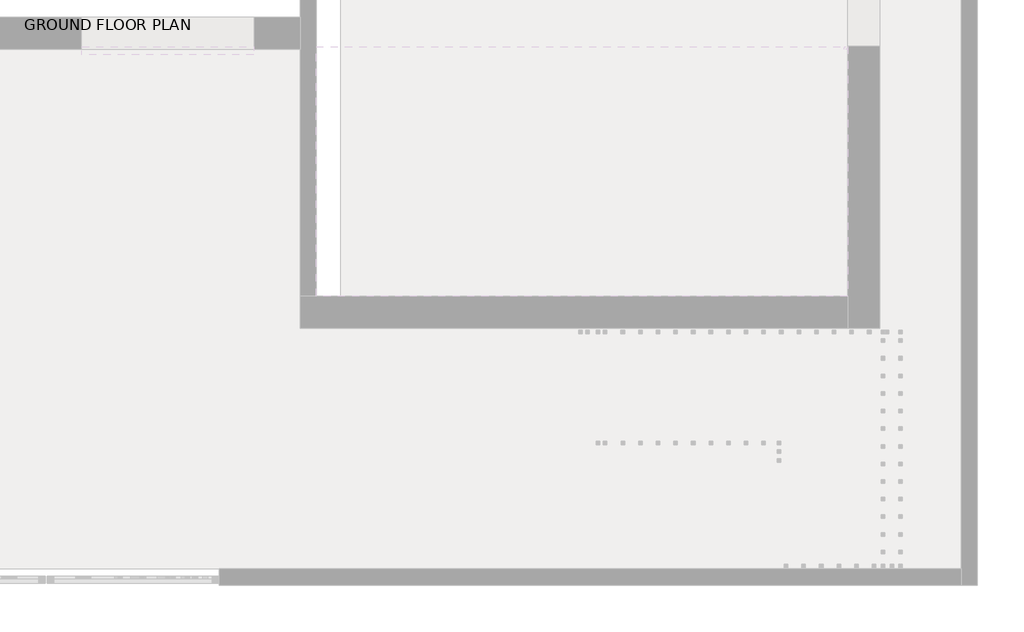
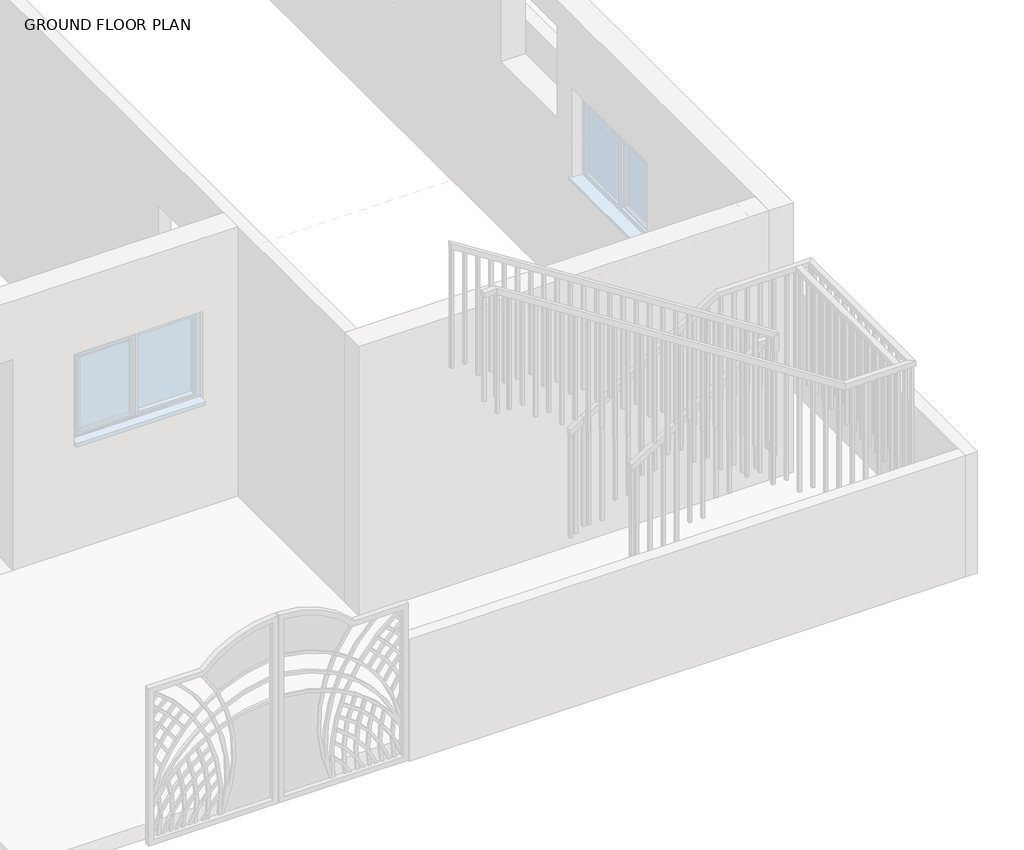
# One storey, part 17 of 23: 2 railings.
"""IFC4 building model written with IfcOpenShell, lengths in millimetres."""

from ifc_helpers import new_model, si_unit, frame, origin, place, context, project, spatial, polyline, outline, extrude, faceted_brep, element, save

model = new_model("IFC4")

# Units and contexts
model_context = context("Model", 3, world=origin())
ifc_project = project(units=[si_unit("LENGTHUNIT", "METRE", prefix="MILLI")], contexts=[model_context])

# Site, building, storey
site = spatial("IfcSite", under=ifc_project)
building = spatial("IfcBuilding", under=site)
storey = spatial("IfcBuildingStorey", under=building, Name="GROUND FLOOR PLAN", Elevation=487.68)

# Railings
placement = place(None, origin())
element("IfcRailing", 1, ObjectType="1100mm", at=placement, inside=storey, context=model_context, shape_type="SolidModel", body=[
    faceted_brep([(-8805.870786, -10220.0521308, 1832.3649576), (-8805.870786, -10220.0521308, 1773.007357), (-8805.870786, -10270.0521308, 1773.007357), (-8805.870786, -10270.0521308, 1832.3649576), (-7409.7306254, -10220.0521308, 2725.6), (-7395.1045513, -10220.0521308, 2675.6), (-7395.1045513, -10270.0521308, 2675.6), (-7409.7306254, -10270.0521308, 2725.6), (-6621.5344696, -10220.0521308, 2725.6), (-6621.5344696, -10220.0521308, 2675.6), (-6671.5344696, -10270.0521308, 2675.6), (-6671.5344696, -10270.0521308, 2725.6), (-6621.5344696, -11933.6860066, 2725.6), (-6621.5344696, -11933.6860066, 2675.6), (-6671.5344696, -11883.6860066, 2675.6), (-6671.5344696, -11883.6860066, 2725.6), (-7155.718398, -11933.6860066, 2725.6), (-7170.3479429, -11933.6860066, 2675.6), (-7170.3479429, -11883.6860066, 2675.6), (-7155.718398, -11883.6860066, 2725.6), (-10457.8773536, -11933.6860066, 4838.88), (-10472.5068984, -11933.6860066, 4788.88), (-10472.5068984, -11883.6860066, 4788.88), (-10457.8773536, -11883.6860066, 4838.88), (-10583.5985666, -11933.6860066, 4838.88), (-10583.5985666, -11883.6860066, 4838.88), (-10583.5985666, -11883.6860066, 4788.88), (-10583.5985666, -11933.6860066, 4788.88)], [[[0, 1, 2, 3]], [[1, 0, 4, 5]], [[2, 1, 5, 6]], [[3, 2, 6, 7]], [[0, 3, 7, 4]], [[5, 4, 8, 9]], [[6, 5, 9, 10]], [[7, 6, 10, 11]], [[4, 7, 11, 8]], [[9, 8, 12, 13]], [[10, 9, 13, 14]], [[11, 10, 14, 15]], [[8, 11, 15, 12]], [[13, 12, 16, 17]], [[14, 13, 17, 18]], [[15, 14, 18, 19]], [[12, 15, 19, 16]], [[17, 16, 20, 21]], [[18, 17, 21, 22]], [[19, 18, 22, 23]], [[16, 19, 23, 20]], [[24, 25, 26, 27]], [[21, 20, 24, 27]], [[22, 21, 27, 26]], [[23, 22, 26, 25]], [[20, 23, 25, 24]]]),
    extrude(outline(polyline([(-10446.5344696, -11921.1860066), (-10471.5344696, -11921.1860066), (-10471.5344696, -11896.1860066), (-10446.5344696, -11896.1860066), (-10446.5344696, -11921.1860066)])), frame((0.0, 0.0, 3738.88), z_axis=(0.0, 0.0, 1.0), x_axis=(1.0, 0.0, 0.0)), (0.0, 0.0, 1.0), 1050.0),
    extrude(outline(polyline([(4692.2622966, -10321.5344696), (4708.2615264, -10346.5344696), (3576.32, -10346.5344696), (3576.32, -10321.5344696), (4692.2622966, -10321.5344696)])), frame((0.0, -11921.1860066, 0.0), z_axis=(0.0, 1.0, 0.0), x_axis=(0.0, 0.0, 1.0)), (0.0, 0.0, 1.0), 25.0),
    extrude(outline(polyline([(4612.2661476, -10196.5344696), (4628.2653774, -10221.5344696), (3576.32, -10221.5344696), (3576.32, -10196.5344696), (4612.2661476, -10196.5344696)])), frame((0.0, -11921.1860066, 0.0), z_axis=(0.0, 1.0, 0.0), x_axis=(0.0, 0.0, 1.0)), (0.0, 0.0, 1.0), 25.0),
    extrude(outline(polyline([(4532.2699985, -10071.5344696), (4548.2692283, -10096.5344696), (3413.76, -10096.5344696), (3413.76, -10071.5344696), (4532.2699985, -10071.5344696)])), frame((0.0, -11921.1860066, 0.0), z_axis=(0.0, 1.0, 0.0), x_axis=(0.0, 0.0, 1.0)), (0.0, 0.0, 1.0), 25.0),
    extrude(outline(polyline([(4452.2738495, -9946.5344696), (4468.2730793, -9971.5344696), (3413.76, -9971.5344696), (3413.76, -9946.5344696), (4452.2738495, -9946.5344696)])), frame((0.0, -11921.1860066, 0.0), z_axis=(0.0, 1.0, 0.0), x_axis=(0.0, 0.0, 1.0)), (0.0, 0.0, 1.0), 25.0),
    extrude(outline(polyline([(4372.2777004, -9821.5344696), (4388.2769302, -9846.5344696), (3251.2, -9846.5344696), (3251.2, -9821.5344696), (4372.2777004, -9821.5344696)])), frame((0.0, -11921.1860066, 0.0), z_axis=(0.0, 1.0, 0.0), x_axis=(0.0, 0.0, 1.0)), (0.0, 0.0, 1.0), 25.0),
    extrude(outline(polyline([(4292.2815514, -9696.5344696), (4308.2807812, -9721.5344696), (3251.2, -9721.5344696), (3251.2, -9696.5344696), (4292.2815514, -9696.5344696)])), frame((0.0, -11921.1860066, 0.0), z_axis=(0.0, 1.0, 0.0), x_axis=(0.0, 0.0, 1.0)), (0.0, 0.0, 1.0), 25.0),
    extrude(outline(polyline([(4212.2854023, -9571.5344696), (4228.2846321, -9596.5344696), (3088.64, -9596.5344696), (3088.64, -9571.5344696), (4212.2854023, -9571.5344696)])), frame((0.0, -11921.1860066, 0.0), z_axis=(0.0, 1.0, 0.0), x_axis=(0.0, 0.0, 1.0)), (0.0, 0.0, 1.0), 25.0),
    extrude(outline(polyline([(4132.2892533, -9446.5344696), (4148.2884831, -9471.5344696), (3088.64, -9471.5344696), (3088.64, -9446.5344696), (4132.2892533, -9446.5344696)])), frame((0.0, -11921.1860066, 0.0), z_axis=(0.0, 1.0, 0.0), x_axis=(0.0, 0.0, 1.0)), (0.0, 0.0, 1.0), 25.0),
    extrude(outline(polyline([(4052.2931042, -9321.5344696), (4068.292334, -9346.5344696), (2926.08, -9346.5344696), (2926.08, -9321.5344696), (4052.2931042, -9321.5344696)])), frame((0.0, -11921.1860066, 0.0), z_axis=(0.0, 1.0, 0.0), x_axis=(0.0, 0.0, 1.0)), (0.0, 0.0, 1.0), 25.0),
    extrude(outline(polyline([(3972.2969552, -9196.5344696), (3988.296185, -9221.5344696), (2926.08, -9221.5344696), (2926.08, -9196.5344696), (3972.2969552, -9196.5344696)])), frame((0.0, -11921.1860066, 0.0), z_axis=(0.0, 1.0, 0.0), x_axis=(0.0, 0.0, 1.0)), (0.0, 0.0, 1.0), 25.0),
    extrude(outline(polyline([(3892.3008061, -9071.5344696), (3908.3000359, -9096.5344696), (2763.52, -9096.5344696), (2763.52, -9071.5344696), (3892.3008061, -9071.5344696)])), frame((0.0, -11921.1860066, 0.0), z_axis=(0.0, 1.0, 0.0), x_axis=(0.0, 0.0, 1.0)), (0.0, 0.0, 1.0), 25.0),
    extrude(outline(polyline([(3812.3046571, -8946.5344696), (3828.3038869, -8971.5344696), (2763.52, -8971.5344696), (2763.52, -8946.5344696), (3812.3046571, -8946.5344696)])), frame((0.0, -11921.1860066, 0.0), z_axis=(0.0, 1.0, 0.0), x_axis=(0.0, 0.0, 1.0)), (0.0, 0.0, 1.0), 25.0),
    extrude(outline(polyline([(3732.308508, -8821.5344696), (3748.3077378, -8846.5344696), (2600.96, -8846.5344696), (2600.96, -8821.5344696), (3732.308508, -8821.5344696)])), frame((0.0, -11921.1860066, 0.0), z_axis=(0.0, 1.0, 0.0), x_axis=(0.0, 0.0, 1.0)), (0.0, 0.0, 1.0), 25.0),
    extrude(outline(polyline([(3652.312359, -8696.5344696), (3668.3115888, -8721.5344696), (2600.96, -8721.5344696), (2600.96, -8696.5344696), (3652.312359, -8696.5344696)])), frame((0.0, -11921.1860066, 0.0), z_axis=(0.0, 1.0, 0.0), x_axis=(0.0, 0.0, 1.0)), (0.0, 0.0, 1.0), 25.0),
    extrude(outline(polyline([(3572.3162099, -8571.5344696), (3588.3154397, -8596.5344696), (2438.4, -8596.5344696), (2438.4, -8571.5344696), (3572.3162099, -8571.5344696)])), frame((0.0, -11921.1860066, 0.0), z_axis=(0.0, 1.0, 0.0), x_axis=(0.0, 0.0, 1.0)), (0.0, 0.0, 1.0), 25.0),
    extrude(outline(polyline([(3492.3200609, -8446.5344696), (3508.3192907, -8471.5344696), (2438.4, -8471.5344696), (2438.4, -8446.5344696), (3492.3200609, -8446.5344696)])), frame((0.0, -11921.1860066, 0.0), z_axis=(0.0, 1.0, 0.0), x_axis=(0.0, 0.0, 1.0)), (0.0, 0.0, 1.0), 25.0),
    extrude(outline(polyline([(3412.3239118, -8321.5344696), (3428.3231416, -8346.5344696), (2275.84, -8346.5344696), (2275.84, -8321.5344696), (3412.3239118, -8321.5344696)])), frame((0.0, -11921.1860066, 0.0), z_axis=(0.0, 1.0, 0.0), x_axis=(0.0, 0.0, 1.0)), (0.0, 0.0, 1.0), 25.0),
    extrude(outline(polyline([(3332.3277628, -8196.5344696), (3348.3269926, -8221.5344696), (2275.84, -8221.5344696), (2275.84, -8196.5344696), (3332.3277628, -8196.5344696)])), frame((0.0, -11921.1860066, 0.0), z_axis=(0.0, 1.0, 0.0), x_axis=(0.0, 0.0, 1.0)), (0.0, 0.0, 1.0), 25.0),
    extrude(outline(polyline([(3252.3316137, -8071.5344696), (3268.3308435, -8096.5344696), (2113.28, -8096.5344696), (2113.28, -8071.5344696), (3252.3316137, -8071.5344696)])), frame((0.0, -11921.1860066, 0.0), z_axis=(0.0, 1.0, 0.0), x_axis=(0.0, 0.0, 1.0)), (0.0, 0.0, 1.0), 25.0),
    extrude(outline(polyline([(3172.3354647, -7946.5344696), (3188.3346945, -7971.5344696), (2113.28, -7971.5344696), (2113.28, -7946.5344696), (3172.3354647, -7946.5344696)])), frame((0.0, -11921.1860066, 0.0), z_axis=(0.0, 1.0, 0.0), x_axis=(0.0, 0.0, 1.0)), (0.0, 0.0, 1.0), 25.0),
    extrude(outline(polyline([(3092.4129874, -7821.5344696), (3108.4077111, -7846.5344696), (1950.72, -7846.5344696), (1950.72, -7821.5344696), (3092.4129874, -7821.5344696)])), frame((0.0, -11921.1860066, 0.0), z_axis=(0.0, 1.0, 0.0), x_axis=(0.0, 0.0, 1.0)), (0.0, 0.0, 1.0), 25.0),
    extrude(outline(polyline([(3012.4393691, -7696.5344696), (3028.4340928, -7721.5344696), (1950.72, -7721.5344696), (1950.72, -7696.5344696), (3012.4393691, -7696.5344696)])), frame((0.0, -11921.1860066, 0.0), z_axis=(0.0, 1.0, 0.0), x_axis=(0.0, 0.0, 1.0)), (0.0, 0.0, 1.0), 25.0),
    extrude(outline(polyline([(2932.4657508, -7571.5344696), (2948.4604745, -7596.5344696), (1788.16, -7596.5344696), (1788.16, -7571.5344696), (2932.4657508, -7571.5344696)])), frame((0.0, -11921.1860066, 0.0), z_axis=(0.0, 1.0, 0.0), x_axis=(0.0, 0.0, 1.0)), (0.0, 0.0, 1.0), 25.0),
    extrude(outline(polyline([(2852.4921325, -7446.5344696), (2868.4868562, -7471.5344696), (1788.16, -7471.5344696), (1788.16, -7446.5344696), (2852.4921325, -7446.5344696)])), frame((0.0, -11921.1860066, 0.0), z_axis=(0.0, 1.0, 0.0), x_axis=(0.0, 0.0, 1.0)), (0.0, 0.0, 1.0), 25.0),
    extrude(outline(polyline([(2772.3547194, -7321.5344696), (2788.3539492, -7346.5344696), (1625.6, -7346.5344696), (1625.6, -7321.5344696), (2772.3547194, -7321.5344696)])), frame((0.0, -11921.1860066, 0.0), z_axis=(0.0, 1.0, 0.0), x_axis=(0.0, 0.0, 1.0)), (0.0, 0.0, 1.0), 25.0),
    extrude(outline(polyline([(2692.3585703, -7196.5344696), (2708.3578001, -7221.5344696), (1625.6, -7221.5344696), (1625.6, -7196.5344696), (2692.3585703, -7196.5344696)])), frame((0.0, -11921.1860066, 0.0), z_axis=(0.0, 1.0, 0.0), x_axis=(0.0, 0.0, 1.0)), (0.0, 0.0, 1.0), 25.0),
    extrude(outline(polyline([(-7071.5344696, -11921.1860066), (-7096.5344696, -11921.1860066), (-7096.5344696, -11896.1860066), (-7071.5344696, -11896.1860066), (-7071.5344696, -11921.1860066)])), frame((0.0, 0.0, 1625.6), z_axis=(0.0, 0.0, 1.0), x_axis=(1.0, 0.0, 0.0)), (0.0, 0.0, 1.0), 1050.0),
    extrude(outline(polyline([(-6946.5344696, -11921.1860066), (-6971.5344696, -11921.1860066), (-6971.5344696, -11896.1860066), (-6946.5344696, -11896.1860066), (-6946.5344696, -11921.1860066)])), frame((0.0, 0.0, 1625.6), z_axis=(0.0, 0.0, 1.0), x_axis=(1.0, 0.0, 0.0)), (0.0, 0.0, 1.0), 1050.0),
    extrude(outline(polyline([(-6821.5344696, -11921.1860066), (-6846.5344696, -11921.1860066), (-6846.5344696, -11896.1860066), (-6821.5344696, -11896.1860066), (-6821.5344696, -11921.1860066)])), frame((0.0, 0.0, 1625.6), z_axis=(0.0, 0.0, 1.0), x_axis=(1.0, 0.0, 0.0)), (0.0, 0.0, 1.0), 1050.0),
    extrude(outline(polyline([(-6696.5344696, -11921.1860066), (-6721.5344696, -11921.1860066), (-6721.5344696, -11896.1860066), (-6696.5344696, -11896.1860066), (-6696.5344696, -11921.1860066)])), frame((0.0, 0.0, 1625.6), z_axis=(0.0, 0.0, 1.0), x_axis=(1.0, 0.0, 0.0)), (0.0, 0.0, 1.0), 1050.0),
    extrude(outline(polyline([(-6634.0344696, -11795.0521308), (-6634.0344696, -11820.0521308), (-6659.0344696, -11820.0521308), (-6659.0344696, -11795.0521308), (-6634.0344696, -11795.0521308)])), frame((0.0, 0.0, 1625.6), z_axis=(0.0, 0.0, 1.0), x_axis=(1.0, 0.0, 0.0)), (0.0, 0.0, 1.0), 1050.0),
    extrude(outline(polyline([(-6634.0344696, -11670.0521308), (-6634.0344696, -11695.0521308), (-6659.0344696, -11695.0521308), (-6659.0344696, -11670.0521308), (-6634.0344696, -11670.0521308)])), frame((0.0, 0.0, 1625.6), z_axis=(0.0, 0.0, 1.0), x_axis=(1.0, 0.0, 0.0)), (0.0, 0.0, 1.0), 1050.0),
    extrude(outline(polyline([(-6634.0344696, -11545.0521308), (-6634.0344696, -11570.0521308), (-6659.0344696, -11570.0521308), (-6659.0344696, -11545.0521308), (-6634.0344696, -11545.0521308)])), frame((0.0, 0.0, 1625.6), z_axis=(0.0, 0.0, 1.0), x_axis=(1.0, 0.0, 0.0)), (0.0, 0.0, 1.0), 1050.0),
    extrude(outline(polyline([(-6634.0344696, -11420.0521308), (-6634.0344696, -11445.0521308), (-6659.0344696, -11445.0521308), (-6659.0344696, -11420.0521308), (-6634.0344696, -11420.0521308)])), frame((0.0, 0.0, 1625.6), z_axis=(0.0, 0.0, 1.0), x_axis=(1.0, 0.0, 0.0)), (0.0, 0.0, 1.0), 1050.0),
    extrude(outline(polyline([(-6634.0344696, -11295.0521308), (-6634.0344696, -11320.0521308), (-6659.0344696, -11320.0521308), (-6659.0344696, -11295.0521308), (-6634.0344696, -11295.0521308)])), frame((0.0, 0.0, 1625.6), z_axis=(0.0, 0.0, 1.0), x_axis=(1.0, 0.0, 0.0)), (0.0, 0.0, 1.0), 1050.0),
    extrude(outline(polyline([(-6634.0344696, -11170.0521308), (-6634.0344696, -11195.0521308), (-6659.0344696, -11195.0521308), (-6659.0344696, -11170.0521308), (-6634.0344696, -11170.0521308)])), frame((0.0, 0.0, 1625.6), z_axis=(0.0, 0.0, 1.0), x_axis=(1.0, 0.0, 0.0)), (0.0, 0.0, 1.0), 1050.0),
    extrude(outline(polyline([(-6634.0344696, -11045.0521308), (-6634.0344696, -11070.0521308), (-6659.0344696, -11070.0521308), (-6659.0344696, -11045.0521308), (-6634.0344696, -11045.0521308)])), frame((0.0, 0.0, 1625.6), z_axis=(0.0, 0.0, 1.0), x_axis=(1.0, 0.0, 0.0)), (0.0, 0.0, 1.0), 1050.0),
    extrude(outline(polyline([(-6634.0344696, -10920.0521308), (-6634.0344696, -10945.0521308), (-6659.0344696, -10945.0521308), (-6659.0344696, -10920.0521308), (-6634.0344696, -10920.0521308)])), frame((0.0, 0.0, 1625.6), z_axis=(0.0, 0.0, 1.0), x_axis=(1.0, 0.0, 0.0)), (0.0, 0.0, 1.0), 1050.0),
    extrude(outline(polyline([(-6634.0344696, -10795.0521308), (-6634.0344696, -10820.0521308), (-6659.0344696, -10820.0521308), (-6659.0344696, -10795.0521308), (-6634.0344696, -10795.0521308)])), frame((0.0, 0.0, 1625.6), z_axis=(0.0, 0.0, 1.0), x_axis=(1.0, 0.0, 0.0)), (0.0, 0.0, 1.0), 1050.0),
    extrude(outline(polyline([(-6634.0344696, -10670.0521308), (-6634.0344696, -10695.0521308), (-6659.0344696, -10695.0521308), (-6659.0344696, -10670.0521308), (-6634.0344696, -10670.0521308)])), frame((0.0, 0.0, 1625.6), z_axis=(0.0, 0.0, 1.0), x_axis=(1.0, 0.0, 0.0)), (0.0, 0.0, 1.0), 1050.0),
    extrude(outline(polyline([(-6634.0344696, -10545.0521308), (-6634.0344696, -10570.0521308), (-6659.0344696, -10570.0521308), (-6659.0344696, -10545.0521308), (-6634.0344696, -10545.0521308)])), frame((0.0, 0.0, 1625.6), z_axis=(0.0, 0.0, 1.0), x_axis=(1.0, 0.0, 0.0)), (0.0, 0.0, 1.0), 1050.0),
    extrude(outline(polyline([(-6634.0344696, -10420.0521308), (-6634.0344696, -10445.0521308), (-6659.0344696, -10445.0521308), (-6659.0344696, -10420.0521308), (-6634.0344696, -10420.0521308)])), frame((0.0, 0.0, 1625.6), z_axis=(0.0, 0.0, 1.0), x_axis=(1.0, 0.0, 0.0)), (0.0, 0.0, 1.0), 1050.0),
    extrude(outline(polyline([(-6634.0344696, -10295.0521308), (-6634.0344696, -10320.0521308), (-6659.0344696, -10320.0521308), (-6659.0344696, -10295.0521308), (-6634.0344696, -10295.0521308)])), frame((0.0, 0.0, 1625.6), z_axis=(0.0, 0.0, 1.0), x_axis=(1.0, 0.0, 0.0)), (0.0, 0.0, 1.0), 1050.0),
    extrude(outline(polyline([(-6755.870786, -10232.5521308), (-6730.870786, -10232.5521308), (-6730.870786, -10257.5521308), (-6755.870786, -10257.5521308), (-6755.870786, -10232.5521308)])), frame((0.0, 0.0, 1625.6), z_axis=(0.0, 0.0, 1.0), x_axis=(1.0, 0.0, 0.0)), (0.0, 0.0, 1.0), 1050.0),
    extrude(outline(polyline([(-6880.870786, -10232.5521308), (-6855.870786, -10232.5521308), (-6855.870786, -10257.5521308), (-6880.870786, -10257.5521308), (-6880.870786, -10232.5521308)])), frame((0.0, 0.0, 1625.6), z_axis=(0.0, 0.0, 1.0), x_axis=(1.0, 0.0, 0.0)), (0.0, 0.0, 1.0), 1050.0),
    extrude(outline(polyline([(-7005.870786, -10232.5521308), (-6980.870786, -10232.5521308), (-6980.870786, -10257.5521308), (-7005.870786, -10257.5521308), (-7005.870786, -10232.5521308)])), frame((0.0, 0.0, 1625.6), z_axis=(0.0, 0.0, 1.0), x_axis=(1.0, 0.0, 0.0)), (0.0, 0.0, 1.0), 1050.0),
    extrude(outline(polyline([(-7130.870786, -10232.5521308), (-7105.870786, -10232.5521308), (-7105.870786, -10257.5521308), (-7130.870786, -10257.5521308), (-7130.870786, -10232.5521308)])), frame((0.0, 0.0, 1625.6), z_axis=(0.0, 0.0, 1.0), x_axis=(1.0, 0.0, 0.0)), (0.0, 0.0, 1.0), 1050.0),
    extrude(outline(polyline([(-7255.870786, -10232.5521308), (-7230.870786, -10232.5521308), (-7230.870786, -10257.5521308), (-7255.870786, -10257.5521308), (-7255.870786, -10232.5521308)])), frame((0.0, 0.0, 1625.6), z_axis=(0.0, 0.0, 1.0), x_axis=(1.0, 0.0, 0.0)), (0.0, 0.0, 1.0), 1050.0),
    extrude(outline(polyline([(-7380.870786, -10232.5521308), (-7355.870786, -10232.5521308), (-7355.870786, -10257.5521308), (-7380.870786, -10257.5521308), (-7380.870786, -10232.5521308)])), frame((0.0, 0.0, 1625.6), z_axis=(0.0, 0.0, 1.0), x_axis=(1.0, 0.0, 0.0)), (0.0, 0.0, 1.0), 1050.0),
    extrude(outline(polyline([(1463.04, -7505.870786), (1463.04, -7480.870786), (2620.7277111, -7480.870786), (2604.7329874, -7505.870786), (1463.04, -7505.870786)])), frame((0.0, -10257.5521308, 0.0), z_axis=(0.0, 1.0, 0.0), x_axis=(0.0, 0.0, 1.0)), (0.0, 0.0, 1.0), 25.0),
    extrude(outline(polyline([(1463.04, -7630.870786), (1463.04, -7605.870786), (2540.7540928, -7605.870786), (2524.7593691, -7630.870786), (1463.04, -7630.870786)])), frame((0.0, -10257.5521308, 0.0), z_axis=(0.0, 1.0, 0.0), x_axis=(0.0, 0.0, 1.0)), (0.0, 0.0, 1.0), 25.0),
    extrude(outline(polyline([(1300.48, -7755.870786), (1300.48, -7730.870786), (2460.7804745, -7730.870786), (2444.7857508, -7755.870786), (1300.48, -7755.870786)])), frame((0.0, -10257.5521308, 0.0), z_axis=(0.0, 1.0, 0.0), x_axis=(0.0, 0.0, 1.0)), (0.0, 0.0, 1.0), 25.0),
    extrude(outline(polyline([(1300.48, -7880.870786), (1300.48, -7855.870786), (2380.8068562, -7855.870786), (2364.8121325, -7880.870786), (1300.48, -7880.870786)])), frame((0.0, -10257.5521308, 0.0), z_axis=(0.0, 1.0, 0.0), x_axis=(0.0, 0.0, 1.0)), (0.0, 0.0, 1.0), 25.0),
    extrude(outline(polyline([(1137.92, -8005.870786), (1137.92, -7980.870786), (2300.8332379, -7980.870786), (2284.8385142, -8005.870786), (1137.92, -8005.870786)])), frame((0.0, -10257.5521308, 0.0), z_axis=(0.0, 1.0, 0.0), x_axis=(0.0, 0.0, 1.0)), (0.0, 0.0, 1.0), 25.0),
    extrude(outline(polyline([(1137.92, -8130.870786), (1137.92, -8105.870786), (2220.8596196, -8105.870786), (2204.8648959, -8130.870786), (1137.92, -8130.870786)])), frame((0.0, -10257.5521308, 0.0), z_axis=(0.0, 1.0, 0.0), x_axis=(0.0, 0.0, 1.0)), (0.0, 0.0, 1.0), 25.0),
    extrude(outline(polyline([(975.36, -8255.870786), (975.36, -8230.870786), (2140.8860012, -8230.870786), (2124.8912776, -8255.870786), (975.36, -8255.870786)])), frame((0.0, -10257.5521308, 0.0), z_axis=(0.0, 1.0, 0.0), x_axis=(0.0, 0.0, 1.0)), (0.0, 0.0, 1.0), 25.0),
    extrude(outline(polyline([(975.36, -8380.870786), (975.36, -8355.870786), (2060.9123829, -8355.870786), (2044.9176593, -8380.870786), (975.36, -8380.870786)])), frame((0.0, -10257.5521308, 0.0), z_axis=(0.0, 1.0, 0.0), x_axis=(0.0, 0.0, 1.0)), (0.0, 0.0, 1.0), 25.0),
    extrude(outline(polyline([(812.8, -8505.870786), (812.8, -8480.870786), (1980.9387646, -8480.870786), (1964.944041, -8505.870786), (812.8, -8505.870786)])), frame((0.0, -10257.5521308, 0.0), z_axis=(0.0, 1.0, 0.0), x_axis=(0.0, 0.0, 1.0)), (0.0, 0.0, 1.0), 25.0),
    extrude(outline(polyline([(812.8, -8630.870786), (812.8, -8605.870786), (1900.9651463, -8605.870786), (1884.9704227, -8630.870786), (812.8, -8630.870786)])), frame((0.0, -10257.5521308, 0.0), z_axis=(0.0, 1.0, 0.0), x_axis=(0.0, 0.0, 1.0)), (0.0, 0.0, 1.0), 25.0),
    extrude(outline(polyline([(772.3517667, -8755.870786), (772.3517667, -8730.870786), (1820.991528, -8730.870786), (1804.9968044, -8755.870786), (772.3517667, -8755.870786)])), frame((0.0, -10257.5521308, 0.0), z_axis=(0.0, 1.0, 0.0), x_axis=(0.0, 0.0, 1.0)), (0.0, 0.0, 1.0), 25.0),
    extrude(outline(polyline([(-6634.0344696, -11896.1860066), (-6634.0344696, -11921.1860066), (-6659.0344696, -11921.1860066), (-6659.0344696, -11896.1860066), (-6634.0344696, -11896.1860066)])), frame((0.0, 0.0, 1625.6), z_axis=(0.0, 0.0, 1.0), x_axis=(1.0, 0.0, 0.0)), (0.0, 0.0, 1.0), 1050.0),
    extrude(outline(polyline([(-6659.0344696, -10232.5521308), (-6634.0344696, -10232.5521308), (-6634.0344696, -10257.5521308), (-6659.0344696, -10257.5521308), (-6659.0344696, -10232.5521308)])), frame((0.0, 0.0, 1625.6), z_axis=(0.0, 0.0, 1.0), x_axis=(1.0, 0.0, 0.0)), (0.0, 0.0, 1.0), 1050.0),
    extrude(outline(polyline([(-10558.5985666, -11921.1860066), (-10583.5985666, -11921.1860066), (-10583.5985666, -11896.1860066), (-10558.5985666, -11896.1860066), (-10558.5985666, -11921.1860066)])), frame((0.0, 0.0, 3738.88), z_axis=(0.0, 0.0, 1.0), x_axis=(1.0, 0.0, 0.0)), (0.0, 0.0, 1.0), 1050.0),
    extrude(outline(polyline([(740.3623194, -8805.870786), (740.3623194, -8780.870786), (1789.0020807, -8780.870786), (1773.007357, -8805.870786), (740.3623194, -8805.870786)])), frame((0.0, -10257.5521308, 0.0), z_axis=(0.0, 1.0, 0.0), x_axis=(0.0, 0.0, 1.0)), (0.0, 0.0, 1.0), 25.0),
])
element("IfcRailing", 2, ObjectType="1100mm", at=placement, inside=storey, context=model_context, shape_type="SolidModel", body=[
    faceted_brep([(-8805.870786, -10220.0521308, 1832.3649576), (-8805.870786, -10220.0521308, 1773.007357), (-8805.870786, -10270.0521308, 1773.007357), (-8805.870786, -10270.0521308, 1832.3649576), (-7409.7306254, -10220.0521308, 2725.6), (-7395.1045513, -10220.0521308, 2675.6), (-7395.1045513, -10270.0521308, 2675.6), (-7409.7306254, -10270.0521308, 2725.6), (-6621.5344696, -10220.0521308, 2725.6), (-6621.5344696, -10220.0521308, 2675.6), (-6671.5344696, -10270.0521308, 2675.6), (-6671.5344696, -10270.0521308, 2725.6), (-6621.5344696, -11933.6860066, 2725.6), (-6621.5344696, -11933.6860066, 2675.6), (-6671.5344696, -11883.6860066, 2675.6), (-6671.5344696, -11883.6860066, 2725.6), (-7155.718398, -11933.6860066, 2725.6), (-7170.3479429, -11933.6860066, 2675.6), (-7170.3479429, -11883.6860066, 2675.6), (-7155.718398, -11883.6860066, 2725.6), (-10457.8773536, -11933.6860066, 4838.88), (-10472.5068984, -11933.6860066, 4788.88), (-10472.5068984, -11883.6860066, 4788.88), (-10457.8773536, -11883.6860066, 4838.88), (-10583.5985666, -11933.6860066, 4838.88), (-10583.5985666, -11883.6860066, 4838.88), (-10583.5985666, -11883.6860066, 4788.88), (-10583.5985666, -11933.6860066, 4788.88)], [[[0, 1, 2, 3]], [[1, 0, 4, 5]], [[2, 1, 5, 6]], [[3, 2, 6, 7]], [[0, 3, 7, 4]], [[5, 4, 8, 9]], [[6, 5, 9, 10]], [[7, 6, 10, 11]], [[4, 7, 11, 8]], [[9, 8, 12, 13]], [[10, 9, 13, 14]], [[11, 10, 14, 15]], [[8, 11, 15, 12]], [[13, 12, 16, 17]], [[14, 13, 17, 18]], [[15, 14, 18, 19]], [[12, 15, 19, 16]], [[17, 16, 20, 21]], [[18, 17, 21, 22]], [[19, 18, 22, 23]], [[16, 19, 23, 20]], [[24, 25, 26, 27]], [[21, 20, 24, 27]], [[22, 21, 27, 26]], [[23, 22, 26, 25]], [[20, 23, 25, 24]]]),
    extrude(outline(polyline([(-10446.5344696, -11921.1860066), (-10471.5344696, -11921.1860066), (-10471.5344696, -11896.1860066), (-10446.5344696, -11896.1860066), (-10446.5344696, -11921.1860066)])), frame((0.0, 0.0, 3738.88), z_axis=(0.0, 0.0, 1.0), x_axis=(1.0, 0.0, 0.0)), (0.0, 0.0, 1.0), 1050.0),
    extrude(outline(polyline([(4692.2622966, -10321.5344696), (4708.2615264, -10346.5344696), (3576.32, -10346.5344696), (3576.32, -10321.5344696), (4692.2622966, -10321.5344696)])), frame((0.0, -11921.1860066, 0.0), z_axis=(0.0, 1.0, 0.0), x_axis=(0.0, 0.0, 1.0)), (0.0, 0.0, 1.0), 25.0),
    extrude(outline(polyline([(4612.2661476, -10196.5344696), (4628.2653774, -10221.5344696), (3576.32, -10221.5344696), (3576.32, -10196.5344696), (4612.2661476, -10196.5344696)])), frame((0.0, -11921.1860066, 0.0), z_axis=(0.0, 1.0, 0.0), x_axis=(0.0, 0.0, 1.0)), (0.0, 0.0, 1.0), 25.0),
    extrude(outline(polyline([(4532.2699985, -10071.5344696), (4548.2692283, -10096.5344696), (3413.76, -10096.5344696), (3413.76, -10071.5344696), (4532.2699985, -10071.5344696)])), frame((0.0, -11921.1860066, 0.0), z_axis=(0.0, 1.0, 0.0), x_axis=(0.0, 0.0, 1.0)), (0.0, 0.0, 1.0), 25.0),
    extrude(outline(polyline([(4452.2738495, -9946.5344696), (4468.2730793, -9971.5344696), (3413.76, -9971.5344696), (3413.76, -9946.5344696), (4452.2738495, -9946.5344696)])), frame((0.0, -11921.1860066, 0.0), z_axis=(0.0, 1.0, 0.0), x_axis=(0.0, 0.0, 1.0)), (0.0, 0.0, 1.0), 25.0),
    extrude(outline(polyline([(4372.2777004, -9821.5344696), (4388.2769302, -9846.5344696), (3251.2, -9846.5344696), (3251.2, -9821.5344696), (4372.2777004, -9821.5344696)])), frame((0.0, -11921.1860066, 0.0), z_axis=(0.0, 1.0, 0.0), x_axis=(0.0, 0.0, 1.0)), (0.0, 0.0, 1.0), 25.0),
    extrude(outline(polyline([(4292.2815514, -9696.5344696), (4308.2807812, -9721.5344696), (3251.2, -9721.5344696), (3251.2, -9696.5344696), (4292.2815514, -9696.5344696)])), frame((0.0, -11921.1860066, 0.0), z_axis=(0.0, 1.0, 0.0), x_axis=(0.0, 0.0, 1.0)), (0.0, 0.0, 1.0), 25.0),
    extrude(outline(polyline([(4212.2854023, -9571.5344696), (4228.2846321, -9596.5344696), (3088.64, -9596.5344696), (3088.64, -9571.5344696), (4212.2854023, -9571.5344696)])), frame((0.0, -11921.1860066, 0.0), z_axis=(0.0, 1.0, 0.0), x_axis=(0.0, 0.0, 1.0)), (0.0, 0.0, 1.0), 25.0),
    extrude(outline(polyline([(4132.2892533, -9446.5344696), (4148.2884831, -9471.5344696), (3088.64, -9471.5344696), (3088.64, -9446.5344696), (4132.2892533, -9446.5344696)])), frame((0.0, -11921.1860066, 0.0), z_axis=(0.0, 1.0, 0.0), x_axis=(0.0, 0.0, 1.0)), (0.0, 0.0, 1.0), 25.0),
    extrude(outline(polyline([(4052.2931042, -9321.5344696), (4068.292334, -9346.5344696), (2926.08, -9346.5344696), (2926.08, -9321.5344696), (4052.2931042, -9321.5344696)])), frame((0.0, -11921.1860066, 0.0), z_axis=(0.0, 1.0, 0.0), x_axis=(0.0, 0.0, 1.0)), (0.0, 0.0, 1.0), 25.0),
    extrude(outline(polyline([(3972.2969552, -9196.5344696), (3988.296185, -9221.5344696), (2926.08, -9221.5344696), (2926.08, -9196.5344696), (3972.2969552, -9196.5344696)])), frame((0.0, -11921.1860066, 0.0), z_axis=(0.0, 1.0, 0.0), x_axis=(0.0, 0.0, 1.0)), (0.0, 0.0, 1.0), 25.0),
    extrude(outline(polyline([(3892.3008061, -9071.5344696), (3908.3000359, -9096.5344696), (2763.52, -9096.5344696), (2763.52, -9071.5344696), (3892.3008061, -9071.5344696)])), frame((0.0, -11921.1860066, 0.0), z_axis=(0.0, 1.0, 0.0), x_axis=(0.0, 0.0, 1.0)), (0.0, 0.0, 1.0), 25.0),
    extrude(outline(polyline([(3812.3046571, -8946.5344696), (3828.3038869, -8971.5344696), (2763.52, -8971.5344696), (2763.52, -8946.5344696), (3812.3046571, -8946.5344696)])), frame((0.0, -11921.1860066, 0.0), z_axis=(0.0, 1.0, 0.0), x_axis=(0.0, 0.0, 1.0)), (0.0, 0.0, 1.0), 25.0),
    extrude(outline(polyline([(3732.308508, -8821.5344696), (3748.3077378, -8846.5344696), (2600.96, -8846.5344696), (2600.96, -8821.5344696), (3732.308508, -8821.5344696)])), frame((0.0, -11921.1860066, 0.0), z_axis=(0.0, 1.0, 0.0), x_axis=(0.0, 0.0, 1.0)), (0.0, 0.0, 1.0), 25.0),
    extrude(outline(polyline([(3652.312359, -8696.5344696), (3668.3115888, -8721.5344696), (2600.96, -8721.5344696), (2600.96, -8696.5344696), (3652.312359, -8696.5344696)])), frame((0.0, -11921.1860066, 0.0), z_axis=(0.0, 1.0, 0.0), x_axis=(0.0, 0.0, 1.0)), (0.0, 0.0, 1.0), 25.0),
    extrude(outline(polyline([(3572.3162099, -8571.5344696), (3588.3154397, -8596.5344696), (2438.4, -8596.5344696), (2438.4, -8571.5344696), (3572.3162099, -8571.5344696)])), frame((0.0, -11921.1860066, 0.0), z_axis=(0.0, 1.0, 0.0), x_axis=(0.0, 0.0, 1.0)), (0.0, 0.0, 1.0), 25.0),
    extrude(outline(polyline([(3492.3200609, -8446.5344696), (3508.3192907, -8471.5344696), (2438.4, -8471.5344696), (2438.4, -8446.5344696), (3492.3200609, -8446.5344696)])), frame((0.0, -11921.1860066, 0.0), z_axis=(0.0, 1.0, 0.0), x_axis=(0.0, 0.0, 1.0)), (0.0, 0.0, 1.0), 25.0),
    extrude(outline(polyline([(3412.3239118, -8321.5344696), (3428.3231416, -8346.5344696), (2275.84, -8346.5344696), (2275.84, -8321.5344696), (3412.3239118, -8321.5344696)])), frame((0.0, -11921.1860066, 0.0), z_axis=(0.0, 1.0, 0.0), x_axis=(0.0, 0.0, 1.0)), (0.0, 0.0, 1.0), 25.0),
    extrude(outline(polyline([(3332.3277628, -8196.5344696), (3348.3269926, -8221.5344696), (2275.84, -8221.5344696), (2275.84, -8196.5344696), (3332.3277628, -8196.5344696)])), frame((0.0, -11921.1860066, 0.0), z_axis=(0.0, 1.0, 0.0), x_axis=(0.0, 0.0, 1.0)), (0.0, 0.0, 1.0), 25.0),
    extrude(outline(polyline([(3252.3316137, -8071.5344696), (3268.3308435, -8096.5344696), (2113.28, -8096.5344696), (2113.28, -8071.5344696), (3252.3316137, -8071.5344696)])), frame((0.0, -11921.1860066, 0.0), z_axis=(0.0, 1.0, 0.0), x_axis=(0.0, 0.0, 1.0)), (0.0, 0.0, 1.0), 25.0),
    extrude(outline(polyline([(3172.3354647, -7946.5344696), (3188.3346945, -7971.5344696), (2113.28, -7971.5344696), (2113.28, -7946.5344696), (3172.3354647, -7946.5344696)])), frame((0.0, -11921.1860066, 0.0), z_axis=(0.0, 1.0, 0.0), x_axis=(0.0, 0.0, 1.0)), (0.0, 0.0, 1.0), 25.0),
    extrude(outline(polyline([(3092.4129874, -7821.5344696), (3108.4077111, -7846.5344696), (1950.72, -7846.5344696), (1950.72, -7821.5344696), (3092.4129874, -7821.5344696)])), frame((0.0, -11921.1860066, 0.0), z_axis=(0.0, 1.0, 0.0), x_axis=(0.0, 0.0, 1.0)), (0.0, 0.0, 1.0), 25.0),
    extrude(outline(polyline([(3012.4393691, -7696.5344696), (3028.4340928, -7721.5344696), (1950.72, -7721.5344696), (1950.72, -7696.5344696), (3012.4393691, -7696.5344696)])), frame((0.0, -11921.1860066, 0.0), z_axis=(0.0, 1.0, 0.0), x_axis=(0.0, 0.0, 1.0)), (0.0, 0.0, 1.0), 25.0),
    extrude(outline(polyline([(2932.4657508, -7571.5344696), (2948.4604745, -7596.5344696), (1788.16, -7596.5344696), (1788.16, -7571.5344696), (2932.4657508, -7571.5344696)])), frame((0.0, -11921.1860066, 0.0), z_axis=(0.0, 1.0, 0.0), x_axis=(0.0, 0.0, 1.0)), (0.0, 0.0, 1.0), 25.0),
    extrude(outline(polyline([(2852.4921325, -7446.5344696), (2868.4868562, -7471.5344696), (1788.16, -7471.5344696), (1788.16, -7446.5344696), (2852.4921325, -7446.5344696)])), frame((0.0, -11921.1860066, 0.0), z_axis=(0.0, 1.0, 0.0), x_axis=(0.0, 0.0, 1.0)), (0.0, 0.0, 1.0), 25.0),
    extrude(outline(polyline([(2772.3547194, -7321.5344696), (2788.3539492, -7346.5344696), (1625.6, -7346.5344696), (1625.6, -7321.5344696), (2772.3547194, -7321.5344696)])), frame((0.0, -11921.1860066, 0.0), z_axis=(0.0, 1.0, 0.0), x_axis=(0.0, 0.0, 1.0)), (0.0, 0.0, 1.0), 25.0),
    extrude(outline(polyline([(2692.3585703, -7196.5344696), (2708.3578001, -7221.5344696), (1625.6, -7221.5344696), (1625.6, -7196.5344696), (2692.3585703, -7196.5344696)])), frame((0.0, -11921.1860066, 0.0), z_axis=(0.0, 1.0, 0.0), x_axis=(0.0, 0.0, 1.0)), (0.0, 0.0, 1.0), 25.0),
    extrude(outline(polyline([(-7071.5344696, -11921.1860066), (-7096.5344696, -11921.1860066), (-7096.5344696, -11896.1860066), (-7071.5344696, -11896.1860066), (-7071.5344696, -11921.1860066)])), frame((0.0, 0.0, 1625.6), z_axis=(0.0, 0.0, 1.0), x_axis=(1.0, 0.0, 0.0)), (0.0, 0.0, 1.0), 1050.0),
    extrude(outline(polyline([(-6946.5344696, -11921.1860066), (-6971.5344696, -11921.1860066), (-6971.5344696, -11896.1860066), (-6946.5344696, -11896.1860066), (-6946.5344696, -11921.1860066)])), frame((0.0, 0.0, 1625.6), z_axis=(0.0, 0.0, 1.0), x_axis=(1.0, 0.0, 0.0)), (0.0, 0.0, 1.0), 1050.0),
    extrude(outline(polyline([(-6821.5344696, -11921.1860066), (-6846.5344696, -11921.1860066), (-6846.5344696, -11896.1860066), (-6821.5344696, -11896.1860066), (-6821.5344696, -11921.1860066)])), frame((0.0, 0.0, 1625.6), z_axis=(0.0, 0.0, 1.0), x_axis=(1.0, 0.0, 0.0)), (0.0, 0.0, 1.0), 1050.0),
    extrude(outline(polyline([(-6696.5344696, -11921.1860066), (-6721.5344696, -11921.1860066), (-6721.5344696, -11896.1860066), (-6696.5344696, -11896.1860066), (-6696.5344696, -11921.1860066)])), frame((0.0, 0.0, 1625.6), z_axis=(0.0, 0.0, 1.0), x_axis=(1.0, 0.0, 0.0)), (0.0, 0.0, 1.0), 1050.0),
    extrude(outline(polyline([(-6634.0344696, -11795.0521308), (-6634.0344696, -11820.0521308), (-6659.0344696, -11820.0521308), (-6659.0344696, -11795.0521308), (-6634.0344696, -11795.0521308)])), frame((0.0, 0.0, 1625.6), z_axis=(0.0, 0.0, 1.0), x_axis=(1.0, 0.0, 0.0)), (0.0, 0.0, 1.0), 1050.0),
    extrude(outline(polyline([(-6634.0344696, -11670.0521308), (-6634.0344696, -11695.0521308), (-6659.0344696, -11695.0521308), (-6659.0344696, -11670.0521308), (-6634.0344696, -11670.0521308)])), frame((0.0, 0.0, 1625.6), z_axis=(0.0, 0.0, 1.0), x_axis=(1.0, 0.0, 0.0)), (0.0, 0.0, 1.0), 1050.0),
    extrude(outline(polyline([(-6634.0344696, -11545.0521308), (-6634.0344696, -11570.0521308), (-6659.0344696, -11570.0521308), (-6659.0344696, -11545.0521308), (-6634.0344696, -11545.0521308)])), frame((0.0, 0.0, 1625.6), z_axis=(0.0, 0.0, 1.0), x_axis=(1.0, 0.0, 0.0)), (0.0, 0.0, 1.0), 1050.0),
    extrude(outline(polyline([(-6634.0344696, -11420.0521308), (-6634.0344696, -11445.0521308), (-6659.0344696, -11445.0521308), (-6659.0344696, -11420.0521308), (-6634.0344696, -11420.0521308)])), frame((0.0, 0.0, 1625.6), z_axis=(0.0, 0.0, 1.0), x_axis=(1.0, 0.0, 0.0)), (0.0, 0.0, 1.0), 1050.0),
    extrude(outline(polyline([(-6634.0344696, -11295.0521308), (-6634.0344696, -11320.0521308), (-6659.0344696, -11320.0521308), (-6659.0344696, -11295.0521308), (-6634.0344696, -11295.0521308)])), frame((0.0, 0.0, 1625.6), z_axis=(0.0, 0.0, 1.0), x_axis=(1.0, 0.0, 0.0)), (0.0, 0.0, 1.0), 1050.0),
    extrude(outline(polyline([(-6634.0344696, -11170.0521308), (-6634.0344696, -11195.0521308), (-6659.0344696, -11195.0521308), (-6659.0344696, -11170.0521308), (-6634.0344696, -11170.0521308)])), frame((0.0, 0.0, 1625.6), z_axis=(0.0, 0.0, 1.0), x_axis=(1.0, 0.0, 0.0)), (0.0, 0.0, 1.0), 1050.0),
    extrude(outline(polyline([(-6634.0344696, -11045.0521308), (-6634.0344696, -11070.0521308), (-6659.0344696, -11070.0521308), (-6659.0344696, -11045.0521308), (-6634.0344696, -11045.0521308)])), frame((0.0, 0.0, 1625.6), z_axis=(0.0, 0.0, 1.0), x_axis=(1.0, 0.0, 0.0)), (0.0, 0.0, 1.0), 1050.0),
    extrude(outline(polyline([(-6634.0344696, -10920.0521308), (-6634.0344696, -10945.0521308), (-6659.0344696, -10945.0521308), (-6659.0344696, -10920.0521308), (-6634.0344696, -10920.0521308)])), frame((0.0, 0.0, 1625.6), z_axis=(0.0, 0.0, 1.0), x_axis=(1.0, 0.0, 0.0)), (0.0, 0.0, 1.0), 1050.0),
    extrude(outline(polyline([(-6634.0344696, -10795.0521308), (-6634.0344696, -10820.0521308), (-6659.0344696, -10820.0521308), (-6659.0344696, -10795.0521308), (-6634.0344696, -10795.0521308)])), frame((0.0, 0.0, 1625.6), z_axis=(0.0, 0.0, 1.0), x_axis=(1.0, 0.0, 0.0)), (0.0, 0.0, 1.0), 1050.0),
    extrude(outline(polyline([(-6634.0344696, -10670.0521308), (-6634.0344696, -10695.0521308), (-6659.0344696, -10695.0521308), (-6659.0344696, -10670.0521308), (-6634.0344696, -10670.0521308)])), frame((0.0, 0.0, 1625.6), z_axis=(0.0, 0.0, 1.0), x_axis=(1.0, 0.0, 0.0)), (0.0, 0.0, 1.0), 1050.0),
    extrude(outline(polyline([(-6634.0344696, -10545.0521308), (-6634.0344696, -10570.0521308), (-6659.0344696, -10570.0521308), (-6659.0344696, -10545.0521308), (-6634.0344696, -10545.0521308)])), frame((0.0, 0.0, 1625.6), z_axis=(0.0, 0.0, 1.0), x_axis=(1.0, 0.0, 0.0)), (0.0, 0.0, 1.0), 1050.0),
    extrude(outline(polyline([(-6634.0344696, -10420.0521308), (-6634.0344696, -10445.0521308), (-6659.0344696, -10445.0521308), (-6659.0344696, -10420.0521308), (-6634.0344696, -10420.0521308)])), frame((0.0, 0.0, 1625.6), z_axis=(0.0, 0.0, 1.0), x_axis=(1.0, 0.0, 0.0)), (0.0, 0.0, 1.0), 1050.0),
    extrude(outline(polyline([(-6634.0344696, -10295.0521308), (-6634.0344696, -10320.0521308), (-6659.0344696, -10320.0521308), (-6659.0344696, -10295.0521308), (-6634.0344696, -10295.0521308)])), frame((0.0, 0.0, 1625.6), z_axis=(0.0, 0.0, 1.0), x_axis=(1.0, 0.0, 0.0)), (0.0, 0.0, 1.0), 1050.0),
    extrude(outline(polyline([(-6755.870786, -10232.5521308), (-6730.870786, -10232.5521308), (-6730.870786, -10257.5521308), (-6755.870786, -10257.5521308), (-6755.870786, -10232.5521308)])), frame((0.0, 0.0, 1625.6), z_axis=(0.0, 0.0, 1.0), x_axis=(1.0, 0.0, 0.0)), (0.0, 0.0, 1.0), 1050.0),
    extrude(outline(polyline([(-6880.870786, -10232.5521308), (-6855.870786, -10232.5521308), (-6855.870786, -10257.5521308), (-6880.870786, -10257.5521308), (-6880.870786, -10232.5521308)])), frame((0.0, 0.0, 1625.6), z_axis=(0.0, 0.0, 1.0), x_axis=(1.0, 0.0, 0.0)), (0.0, 0.0, 1.0), 1050.0),
    extrude(outline(polyline([(-7005.870786, -10232.5521308), (-6980.870786, -10232.5521308), (-6980.870786, -10257.5521308), (-7005.870786, -10257.5521308), (-7005.870786, -10232.5521308)])), frame((0.0, 0.0, 1625.6), z_axis=(0.0, 0.0, 1.0), x_axis=(1.0, 0.0, 0.0)), (0.0, 0.0, 1.0), 1050.0),
    extrude(outline(polyline([(-7130.870786, -10232.5521308), (-7105.870786, -10232.5521308), (-7105.870786, -10257.5521308), (-7130.870786, -10257.5521308), (-7130.870786, -10232.5521308)])), frame((0.0, 0.0, 1625.6), z_axis=(0.0, 0.0, 1.0), x_axis=(1.0, 0.0, 0.0)), (0.0, 0.0, 1.0), 1050.0),
    extrude(outline(polyline([(-7255.870786, -10232.5521308), (-7230.870786, -10232.5521308), (-7230.870786, -10257.5521308), (-7255.870786, -10257.5521308), (-7255.870786, -10232.5521308)])), frame((0.0, 0.0, 1625.6), z_axis=(0.0, 0.0, 1.0), x_axis=(1.0, 0.0, 0.0)), (0.0, 0.0, 1.0), 1050.0),
    extrude(outline(polyline([(-7380.870786, -10232.5521308), (-7355.870786, -10232.5521308), (-7355.870786, -10257.5521308), (-7380.870786, -10257.5521308), (-7380.870786, -10232.5521308)])), frame((0.0, 0.0, 1625.6), z_axis=(0.0, 0.0, 1.0), x_axis=(1.0, 0.0, 0.0)), (0.0, 0.0, 1.0), 1050.0),
    extrude(outline(polyline([(1463.04, -7505.870786), (1463.04, -7480.870786), (2620.7277111, -7480.870786), (2604.7329874, -7505.870786), (1463.04, -7505.870786)])), frame((0.0, -10257.5521308, 0.0), z_axis=(0.0, 1.0, 0.0), x_axis=(0.0, 0.0, 1.0)), (0.0, 0.0, 1.0), 25.0),
    extrude(outline(polyline([(1463.04, -7630.870786), (1463.04, -7605.870786), (2540.7540928, -7605.870786), (2524.7593691, -7630.870786), (1463.04, -7630.870786)])), frame((0.0, -10257.5521308, 0.0), z_axis=(0.0, 1.0, 0.0), x_axis=(0.0, 0.0, 1.0)), (0.0, 0.0, 1.0), 25.0),
    extrude(outline(polyline([(1300.48, -7755.870786), (1300.48, -7730.870786), (2460.7804745, -7730.870786), (2444.7857508, -7755.870786), (1300.48, -7755.870786)])), frame((0.0, -10257.5521308, 0.0), z_axis=(0.0, 1.0, 0.0), x_axis=(0.0, 0.0, 1.0)), (0.0, 0.0, 1.0), 25.0),
    extrude(outline(polyline([(1300.48, -7880.870786), (1300.48, -7855.870786), (2380.8068562, -7855.870786), (2364.8121325, -7880.870786), (1300.48, -7880.870786)])), frame((0.0, -10257.5521308, 0.0), z_axis=(0.0, 1.0, 0.0), x_axis=(0.0, 0.0, 1.0)), (0.0, 0.0, 1.0), 25.0),
    extrude(outline(polyline([(1137.92, -8005.870786), (1137.92, -7980.870786), (2300.8332379, -7980.870786), (2284.8385142, -8005.870786), (1137.92, -8005.870786)])), frame((0.0, -10257.5521308, 0.0), z_axis=(0.0, 1.0, 0.0), x_axis=(0.0, 0.0, 1.0)), (0.0, 0.0, 1.0), 25.0),
    extrude(outline(polyline([(1137.92, -8130.870786), (1137.92, -8105.870786), (2220.8596196, -8105.870786), (2204.8648959, -8130.870786), (1137.92, -8130.870786)])), frame((0.0, -10257.5521308, 0.0), z_axis=(0.0, 1.0, 0.0), x_axis=(0.0, 0.0, 1.0)), (0.0, 0.0, 1.0), 25.0),
    extrude(outline(polyline([(975.36, -8255.870786), (975.36, -8230.870786), (2140.8860012, -8230.870786), (2124.8912776, -8255.870786), (975.36, -8255.870786)])), frame((0.0, -10257.5521308, 0.0), z_axis=(0.0, 1.0, 0.0), x_axis=(0.0, 0.0, 1.0)), (0.0, 0.0, 1.0), 25.0),
    extrude(outline(polyline([(975.36, -8380.870786), (975.36, -8355.870786), (2060.9123829, -8355.870786), (2044.9176593, -8380.870786), (975.36, -8380.870786)])), frame((0.0, -10257.5521308, 0.0), z_axis=(0.0, 1.0, 0.0), x_axis=(0.0, 0.0, 1.0)), (0.0, 0.0, 1.0), 25.0),
    extrude(outline(polyline([(812.8, -8505.870786), (812.8, -8480.870786), (1980.9387646, -8480.870786), (1964.944041, -8505.870786), (812.8, -8505.870786)])), frame((0.0, -10257.5521308, 0.0), z_axis=(0.0, 1.0, 0.0), x_axis=(0.0, 0.0, 1.0)), (0.0, 0.0, 1.0), 25.0),
    extrude(outline(polyline([(812.8, -8630.870786), (812.8, -8605.870786), (1900.9651463, -8605.870786), (1884.9704227, -8630.870786), (812.8, -8630.870786)])), frame((0.0, -10257.5521308, 0.0), z_axis=(0.0, 1.0, 0.0), x_axis=(0.0, 0.0, 1.0)), (0.0, 0.0, 1.0), 25.0),
    extrude(outline(polyline([(772.3517667, -8755.870786), (772.3517667, -8730.870786), (1820.991528, -8730.870786), (1804.9968044, -8755.870786), (772.3517667, -8755.870786)])), frame((0.0, -10257.5521308, 0.0), z_axis=(0.0, 1.0, 0.0), x_axis=(0.0, 0.0, 1.0)), (0.0, 0.0, 1.0), 25.0),
    extrude(outline(polyline([(-6634.0344696, -11896.1860066), (-6634.0344696, -11921.1860066), (-6659.0344696, -11921.1860066), (-6659.0344696, -11896.1860066), (-6634.0344696, -11896.1860066)])), frame((0.0, 0.0, 1625.6), z_axis=(0.0, 0.0, 1.0), x_axis=(1.0, 0.0, 0.0)), (0.0, 0.0, 1.0), 1050.0),
    extrude(outline(polyline([(-6659.0344696, -10232.5521308), (-6634.0344696, -10232.5521308), (-6634.0344696, -10257.5521308), (-6659.0344696, -10257.5521308), (-6659.0344696, -10232.5521308)])), frame((0.0, 0.0, 1625.6), z_axis=(0.0, 0.0, 1.0), x_axis=(1.0, 0.0, 0.0)), (0.0, 0.0, 1.0), 1050.0),
    extrude(outline(polyline([(-10558.5985666, -11921.1860066), (-10583.5985666, -11921.1860066), (-10583.5985666, -11896.1860066), (-10558.5985666, -11896.1860066), (-10558.5985666, -11921.1860066)])), frame((0.0, 0.0, 3738.88), z_axis=(0.0, 0.0, 1.0), x_axis=(1.0, 0.0, 0.0)), (0.0, 0.0, 1.0), 1050.0),
    extrude(outline(polyline([(740.3623194, -8805.870786), (740.3623194, -8780.870786), (1789.0020807, -8780.870786), (1773.007357, -8805.870786), (740.3623194, -8805.870786)])), frame((0.0, -10257.5521308, 0.0), z_axis=(0.0, 1.0, 0.0), x_axis=(0.0, 0.0, 1.0)), (0.0, 0.0, 1.0), 25.0),
])

save(model, "model.ifc")

# Revit data of these elements
# Type "1100mm"
#   built-in parameter 1008612 = 0.019685 (stored number, unit not read)
#   built-in parameter 1008611 = 0.019685 (stored number, unit not read)
#   built-in parameter 1008609 = 0.902231 (stored number, unit not read)
#   built-in parameter 1008604 = 0.19685 (stored number, unit not read)
#   built-in parameter 1008603 = 0.164042 (stored number, unit not read)
#   Railing Height = 3.608924 ft
#   built-in parameter 1008630 = 2
#   built-in parameter 1008610 = 2
#   built-in parameter 1008608 = 1
#   built-in parameter 1008618 = Baluster_Square : 25mm
# Elements 1, 2 (IfcRailing, "1100mm")
#   Phase Created = New Construction
